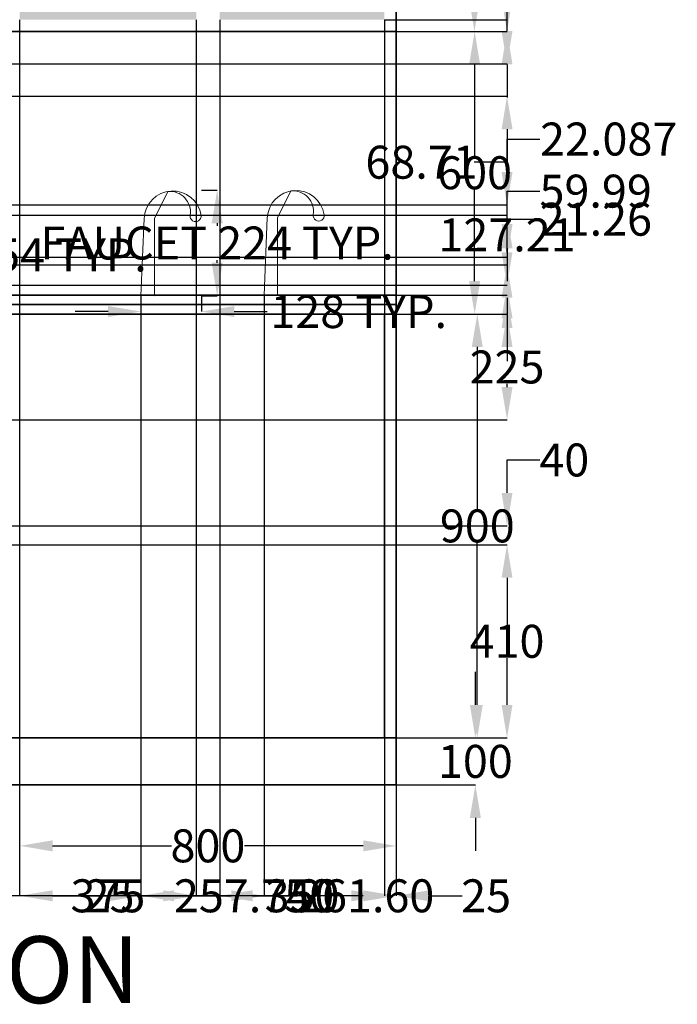
# Model space of a CAD drawing. Units: inches. Extents: x 600 to 5582, y -464 to 3142.
# Tile 8 of 9: x 4185 to 5582, y -464 to 1627. Entities that reach past the tile are written whole.
import ezdxf

# ---------------------------------------------------------------- set-up
doc = ezdxf.new("R2010")
doc.units = ezdxf.units.IN
doc.header["$MEASUREMENT"] = 0
for name, color, linetype, lineweight in [('A-ANNO-DIMS', 2, 'Continuous', 18), ('A-ANNO-TEXT', 7, 'Continuous', 25), ('A-ELEV', 7, 'Continuous', 35), ('A-ELEV-PATT', 252, 'Continuous', 13), ('A-FLOR-FIXT', 8, 'Continuous', 18)]:
    doc.layers.add(name, color=color, linetype=linetype, lineweight=lineweight)
doc.styles.get("Standard").update_dxf_attribs({"font": 'arial.ttf'})
doc.dimstyles.get("Standard").update_dxf_attribs({"dimtxt": 70, "dimasz": 70, "dimexe": 0.18, "dimexo": 0.0625, "dimgap": 0.09, "dimtad": 0, "dimtih": 1, "dimtoh": 1, "dimdec": 0, "dimzin": 0, "dimdsep": 46, "dimtxsty": 'Standard', "dimcen": 0.09, "dimadec": 0, "dimazin": 0, "dimtfac": 1, "dimtdec": 0, "dimtofl": 0, "dimtmove": 0, "dimatfit": 3, "dimfxl": 1, "dimtolj": 1, "dimtzin": 0, "dimarcsym": 0})

# ---------------------------------------------------------------- blocks, each defined once
blk = doc.blocks.new('*D2')
at = {"layer": 'A-ANNO-DIMS', "color": 0, "lineweight": -2, "transparency": 16777216}
for p, q in [((5152.9, 172.4), (5152.9, 242.4)), ((4984.8, 102.4), (5153.1, 102.4)), ((4984.8, 2.4), (5153.1, 2.4)), ((5152.9, -67.6), (5152.9, -137.6))]:
    blk.add_line(p, q, dxfattribs=at)
at = {"layer": 'A-ANNO-DIMS', "color": 0, "transparency": 16777216}
for points in [[(5141.2, 172.4), (5164.6, 172.4), (5152.9, 102.4)], [(5141.2, -67.6), (5164.6, -67.6), (5152.9, 2.4)]]:
    blk.add_solid(points, dxfattribs=at)
at = {"layer": 'Defpoints', "color": 0, "transparency": 16777216}
for p in [(4984.7, 102.4), (4984.7, 2.4), (5152.9, 2.4)]:
    blk.add_point(p, dxfattribs=at)
at = {"layer": 'A-ANNO-DIMS', "color": 0, "transparency": 16777216, "insert": (5152.9, 52.4), "char_height": 70, "attachment_point": 5}
blk.add_mtext('\\A1;100', dxfattribs=at)
blk = doc.blocks.new('*D3')
at = {"layer": 'A-ANNO-DIMS', "color": 0, "lineweight": -2, "transparency": 16777216}
for p, q in [((4984.8, 1002.4), (5157.2, 1002.4)), ((5157, 932.4), (5157, 588.3)), ((5157, 172.4), (5157, 516.6)), ((4984.8, 102.4), (5157.2, 102.4))]:
    blk.add_line(p, q, dxfattribs=at)
at = {"layer": 'A-ANNO-DIMS', "color": 0, "transparency": 16777216}
for points in [[(5145.3, 932.4), (5168.6, 932.4), (5157, 1002.4)], [(5145.3, 172.4), (5168.6, 172.4), (5157, 102.4)]]:
    blk.add_solid(points, dxfattribs=at)
at = {"layer": 'Defpoints', "color": 0, "transparency": 16777216}
for p in [(4984.7, 1002.4), (5157, 1002.4), (4984.7, 102.4)]:
    blk.add_point(p, dxfattribs=at)
at = {"layer": 'A-ANNO-DIMS', "color": 0, "transparency": 16777216, "insert": (5157, 552.4), "char_height": 70, "attachment_point": 5}
blk.add_mtext('\\A1;900', dxfattribs=at)
blk = doc.blocks.new('*D4')
at = {"layer": 'A-ANNO-DIMS', "color": 0, "lineweight": -2, "transparency": 16777216}
for p, q in [((4984.8, 1602.4), (5151.6, 1602.4)), ((5151.4, 1532.4), (5151.4, 1338.3)), ((5151.4, 1072.4), (5151.4, 1266.6)), ((4984.8, 1002.4), (5151.6, 1002.4))]:
    blk.add_line(p, q, dxfattribs=at)
at = {"layer": 'A-ANNO-DIMS', "color": 0, "transparency": 16777216}
for points in [[(5139.7, 1532.4), (5163.1, 1532.4), (5151.4, 1602.4)], [(5139.7, 1072.4), (5163.1, 1072.4), (5151.4, 1002.4)]]:
    blk.add_solid(points, dxfattribs=at)
at = {"layer": 'Defpoints', "color": 0, "transparency": 16777216}
for p in [(4984.7, 1602.4), (4984.7, 1002.4), (5151.4, 1002.4)]:
    blk.add_point(p, dxfattribs=at)
at = {"layer": 'A-ANNO-DIMS', "color": 0, "transparency": 16777216, "insert": (5151.4, 1302.4), "char_height": 70, "attachment_point": 5}
blk.add_mtext('\\A1;600', dxfattribs=at)
blk = doc.blocks.new('*D5')
at = {"layer": 'A-ANNO-DIMS', "color": 0, "lineweight": -2, "transparency": 16777216}
for p, q in [((4984.8, 2352.4), (5151.2, 2352.4)), ((5151, 2282.4), (5151, 2013.3)), ((5151, 1672.4), (5151, 1941.6)), ((4984.8, 1602.4), (5151.2, 1602.4))]:
    blk.add_line(p, q, dxfattribs=at)
at = {"layer": 'A-ANNO-DIMS', "color": 0, "transparency": 16777216}
for points in [[(5139.4, 2282.4), (5162.7, 2282.4), (5151, 2352.4)], [(5139.4, 1672.4), (5162.7, 1672.4), (5151, 1602.4)]]:
    blk.add_solid(points, dxfattribs=at)
at = {"layer": 'Defpoints', "color": 0, "transparency": 16777216}
for p in [(4984.7, 2352.4), (4984.7, 1602.4), (5151, 1602.4)]:
    blk.add_point(p, dxfattribs=at)
at = {"layer": 'A-ANNO-DIMS', "color": 0, "transparency": 16777216, "insert": (5151, 1977.4), "char_height": 70, "attachment_point": 5}
blk.add_mtext('\\A1;750', dxfattribs=at)
blk = doc.blocks.new('*D14')
at = {"layer": 'A-ANNO-DIMS', "color": 0, "lineweight": -2, "transparency": 16777216}
for p, q in [((4184.7, 2.4), (4184.7, -127.2)), ((4984.7, 2.4), (4984.7, -127.2)), ((4254.7, -127), (4507.4, -127)), ((4914.7, -127), (4662.1, -127))]:
    blk.add_line(p, q, dxfattribs=at)
at = {"layer": 'A-ANNO-DIMS', "color": 0, "transparency": 16777216}
for points in [[(4254.7, -115.3), (4254.7, -138.7), (4184.7, -127)], [(4914.7, -115.3), (4914.7, -138.7), (4984.7, -127)]]:
    blk.add_solid(points, dxfattribs=at)
at = {"layer": 'Defpoints', "color": 0, "transparency": 16777216}
for p in [(4184.7, 2.4), (4984.7, 2.4), (4984.7, -127)]:
    blk.add_point(p, dxfattribs=at)
at = {"layer": 'A-ANNO-DIMS', "color": 0, "transparency": 16777216, "insert": (4584.7, -127), "char_height": 70, "attachment_point": 5}
blk.add_mtext('\\A1;800', dxfattribs=at)
blk = doc.blocks.new('FAUCET')
blk.add_lwpolyline([(0.1, 0.4), (6.9, 164.5, -0.907043), (127.6, 171.3, -1.166611), (104.6, 171.3, 0.489908), (56.8, 221.8), (28.6, 164.5), (28.6, 0.4), (0.1, 1.6)], format="xyb")
blk = doc.blocks.new('*D17')
at = {"layer": 'A-ANNO-DIMS', "color": 0, "lineweight": -2, "transparency": 16777216}
for p, q in [((3196.2, 1104.9), (3196.2, 1128.1)), ((3266.2, 1127.9), (3279.8, 1127.9)), ((3349.8, 1104.9), (3349.8, 1128.1)), ((3349.8, 1127.9), (3419.8, 1127.9))]:
    blk.add_line(p, q, dxfattribs=at)
at = {"layer": 'A-ANNO-DIMS', "color": 0, "transparency": 16777216}
for points in [[(3266.2, 1139.5), (3266.2, 1116.2), (3196.2, 1127.9)], [(3279.8, 1139.5), (3279.8, 1116.2), (3349.8, 1127.9)]]:
    blk.add_solid(points, dxfattribs=at)
at = {"layer": 'Defpoints', "color": 0, "transparency": 16777216}
for p in [(3349.8, 1127.9), (3196.2, 1104.9), (3349.8, 1104.9)]:
    blk.add_point(p, dxfattribs=at)
at = {"layer": 'A-ANNO-DIMS', "color": 0, "transparency": 16777216, "insert": (3955.1, 1127.9), "char_height": 70, "attachment_point": 5}
blk.add_mtext('\\A1;HOB BURNER 154 TYP.', dxfattribs=at)
blk = doc.blocks.new('*D19')
at = {"layer": 'A-ANNO-DIMS', "color": 0, "lineweight": -2, "transparency": 16777216}
for p, q in [((4570.8, 1265.2), (4604.5, 1265.2)), ((4604.3, 1195.2), (4604.3, 1189.5)), ((4604.3, 1111.2), (4604.3, 1117)), ((4570.8, 1041.2), (4604.5, 1041.2))]:
    blk.add_line(p, q, dxfattribs=at)
at = {"layer": 'A-ANNO-DIMS', "color": 0, "transparency": 16777216}
for points in [[(4592.7, 1195.2), (4616, 1195.2), (4604.3, 1265.2)], [(4592.7, 1111.2), (4616, 1111.2), (4604.3, 1041.2)]]:
    blk.add_solid(points, dxfattribs=at)
at = {"layer": 'Defpoints', "color": 0, "transparency": 16777216}
for p in [(4570.7, 1265.2), (4604.3, 1265.2), (4570.7, 1041.2)]:
    blk.add_point(p, dxfattribs=at)
at = {"layer": 'A-ANNO-DIMS', "color": 0, "transparency": 16777216, "insert": (4604.3, 1153.2), "char_height": 70, "attachment_point": 5}
blk.add_mtext('\\A1;FAUCET 224 TYP.', dxfattribs=at)
blk = doc.blocks.new('*D20')
at = {"layer": 'A-ANNO-DIMS', "color": 0, "lineweight": -2, "transparency": 16777216}
for p, q in [((4442.5, 1041.2), (4442.5, 1007.5)), ((4570.7, 1041.2), (4570.7, 1007.5)), ((4372.5, 1007.6), (4302.5, 1007.6)), ((4640.7, 1007.6), (4710.7, 1007.6))]:
    blk.add_line(p, q, dxfattribs=at)
at = {"layer": 'A-ANNO-DIMS', "color": 0, "transparency": 16777216}
for points in [[(4372.5, 1019.3), (4372.5, 996), (4442.5, 1007.6)], [(4640.7, 1019.3), (4640.7, 996), (4570.7, 1007.6)]]:
    blk.add_solid(points, dxfattribs=at)
at = {"layer": 'Defpoints', "color": 0, "transparency": 16777216}
for p in [(4442.5, 1041.2), (4570.7, 1041.2), (4570.7, 1007.6)]:
    blk.add_point(p, dxfattribs=at)
at = {"layer": 'A-ANNO-DIMS', "color": 0, "transparency": 16777216, "insert": (4905.1, 1007.6), "char_height": 70, "attachment_point": 5}
blk.add_mtext('\\A1;128 TYP.', dxfattribs=at)
blk = doc.blocks.new('*D21')
at = {"layer": 'A-ANNO-DIMS', "color": 0, "lineweight": -2, "transparency": 16777216}
for p, q in [((1384.7, 2.4), (1384.7, -233.3)), ((4984.7, 2.4), (4984.7, -233.3)), ((1454.7, -233.1), (3080.3, -233.1)), ((4914.7, -233.1), (3289.2, -233.1))]:
    blk.add_line(p, q, dxfattribs=at)
at = {"layer": 'A-ANNO-DIMS', "color": 0, "transparency": 16777216}
for points in [[(1454.7, -221.4), (1454.7, -244.7), (1384.7, -233.1)], [(4914.7, -221.4), (4914.7, -244.7), (4984.7, -233.1)]]:
    blk.add_solid(points, dxfattribs=at)
at = {"layer": 'Defpoints', "color": 0, "transparency": 16777216}
for p in [(1384.7, 2.4), (4984.7, 2.4), (4984.7, -233.1)]:
    blk.add_point(p, dxfattribs=at)
at = {"layer": 'A-ANNO-DIMS', "color": 0, "transparency": 16777216, "insert": (3184.7, -233.1), "char_height": 70, "attachment_point": 5}
blk.add_mtext('\\A1;3600', dxfattribs=at)
blk = doc.blocks.new('*D30')
at = {"layer": 'A-ANNO-DIMS', "color": 0, "lineweight": -2, "transparency": 16777216}
for p, q in [((4159.7, 1627.4), (4159.7, -233.3)), ((4184.7, 1627.4), (4184.7, -233.3)), ((4089.7, -233.1), (4019.7, -233.1)), ((4254.7, -233.1), (4324.7, -233.1))]:
    blk.add_line(p, q, dxfattribs=at)
at = {"layer": 'A-ANNO-DIMS', "color": 0, "transparency": 16777216}
for points in [[(4089.7, -221.4), (4089.7, -244.7), (4159.7, -233.1)], [(4254.7, -221.4), (4254.7, -244.7), (4184.7, -233.1)]]:
    blk.add_solid(points, dxfattribs=at)
at = {"layer": 'Defpoints', "color": 0, "transparency": 16777216}
for p in [(4159.7, 1627.4), (4184.7, 1627.4), (4184.7, -233.1)]:
    blk.add_point(p, dxfattribs=at)
at = {"layer": 'A-ANNO-DIMS', "color": 0, "transparency": 16777216, "insert": (4375.8, -233.1), "char_height": 70, "attachment_point": 5}
blk.add_mtext('\\A1;25', dxfattribs=at)
blk = doc.blocks.new('*D31')
at = {"layer": 'A-ANNO-DIMS', "color": 0, "lineweight": -2, "transparency": 16777216}
for p, q in [((4184.7, 1627.4), (4184.7, -233.3)), ((4559.7, 1627.4), (4559.7, -233.3)), ((4254.7, -233.1), (4294.6, -233.1)), ((4489.7, -233.1), (4449.9, -233.1))]:
    blk.add_line(p, q, dxfattribs=at)
at = {"layer": 'A-ANNO-DIMS', "color": 0, "transparency": 16777216}
for points in [[(4254.7, -221.4), (4254.7, -244.7), (4184.7, -233.1)], [(4489.7, -221.4), (4489.7, -244.7), (4559.7, -233.1)]]:
    blk.add_solid(points, dxfattribs=at)
at = {"layer": 'Defpoints', "color": 0, "transparency": 16777216}
for p in [(4184.7, 1627.4), (4559.7, 1627.4), (4559.7, -233.1)]:
    blk.add_point(p, dxfattribs=at)
at = {"layer": 'A-ANNO-DIMS', "color": 0, "transparency": 16777216, "insert": (4372.2, -233.1), "char_height": 70, "attachment_point": 5}
blk.add_mtext('\\A1;375', dxfattribs=at)
blk = doc.blocks.new('*D32')
at = {"layer": 'A-ANNO-DIMS', "color": 0, "lineweight": -2, "transparency": 16777216}
for p, q in [((4559.7, 1627.4), (4559.7, -233.3)), ((4609.7, 1627.4), (4609.7, -233.3)), ((4489.7, -233.1), (4419.7, -233.1)), ((4679.7, -233.1), (4749.7, -233.1))]:
    blk.add_line(p, q, dxfattribs=at)
at = {"layer": 'A-ANNO-DIMS', "color": 0, "transparency": 16777216}
for points in [[(4489.7, -221.4), (4489.7, -244.7), (4559.7, -233.1)], [(4679.7, -221.4), (4679.7, -244.7), (4609.7, -233.1)]]:
    blk.add_solid(points, dxfattribs=at)
at = {"layer": 'Defpoints', "color": 0, "transparency": 16777216}
for p in [(4559.7, 1627.4), (4609.7, 1627.4), (4609.7, -233.1)]:
    blk.add_point(p, dxfattribs=at)
at = {"layer": 'A-ANNO-DIMS', "color": 0, "transparency": 16777216, "insert": (4799.9, -233.1), "char_height": 70, "attachment_point": 5}
blk.add_mtext('\\A1;50', dxfattribs=at)
blk = doc.blocks.new('*D33')
at = {"layer": 'A-ANNO-DIMS', "color": 0, "lineweight": -2, "transparency": 16777216}
for p, q in [((4609.7, 1627.4), (4609.7, -233.3)), ((4959.7, 1627.4), (4959.7, -233.3)), ((4679.7, -233.1), (4707.5, -233.1)), ((4889.7, -233.1), (4862, -233.1))]:
    blk.add_line(p, q, dxfattribs=at)
at = {"layer": 'A-ANNO-DIMS', "color": 0, "transparency": 16777216}
for points in [[(4679.7, -221.4), (4679.7, -244.7), (4609.7, -233.1)], [(4889.7, -221.4), (4889.7, -244.7), (4959.7, -233.1)]]:
    blk.add_solid(points, dxfattribs=at)
at = {"layer": 'Defpoints', "color": 0, "transparency": 16777216}
for p in [(4609.7, 1627.4), (4959.7, 1627.4), (4959.7, -233.1)]:
    blk.add_point(p, dxfattribs=at)
at = {"layer": 'A-ANNO-DIMS', "color": 0, "transparency": 16777216, "insert": (4784.7, -233.1), "char_height": 70, "attachment_point": 5}
blk.add_mtext('\\A1;350', dxfattribs=at)
blk = doc.blocks.new('*D34')
at = {"layer": 'A-ANNO-DIMS', "color": 0, "lineweight": -2, "transparency": 16777216}
for p, q in [((4959.7, 1627.4), (4959.7, -233.3)), ((4984.7, 1602.4), (4984.7, -233.3)), ((4889.7, -233.1), (4819.7, -233.1)), ((5054.7, -233.1), (5124.7, -233.1))]:
    blk.add_line(p, q, dxfattribs=at)
at = {"layer": 'A-ANNO-DIMS', "color": 0, "transparency": 16777216}
for points in [[(4889.7, -221.4), (4889.7, -244.7), (4959.7, -233.1)], [(5054.7, -221.4), (5054.7, -244.7), (4984.7, -233.1)]]:
    blk.add_solid(points, dxfattribs=at)
at = {"layer": 'Defpoints', "color": 0, "transparency": 16777216}
for p in [(4959.7, 1627.4), (4984.7, 1602.4), (4984.7, -233.1)]:
    blk.add_point(p, dxfattribs=at)
at = {"layer": 'A-ANNO-DIMS', "color": 0, "transparency": 16777216, "insert": (5175.8, -233.1), "char_height": 70, "attachment_point": 5}
blk.add_mtext('\\A1;25', dxfattribs=at)
blk = doc.blocks.new('*D35')
at = {"layer": 'A-ANNO-DIMS', "color": 0, "lineweight": -2, "transparency": 16777216}
for p, q in [((5220.2, 1697.4), (5220.2, 1767.4)), ((5220.2, 1767.4), (5290.2, 1767.4)), ((4959.8, 1627.4), (5220.4, 1627.4)), ((4984.8, 1602.4), (5220.4, 1602.4)), ((5220.2, 1532.4), (5220.2, 1462.4))]:
    blk.add_line(p, q, dxfattribs=at)
at = {"layer": 'A-ANNO-DIMS', "color": 0, "transparency": 16777216}
for points in [[(5208.6, 1697.4), (5231.9, 1697.4), (5220.2, 1627.4)], [(5208.6, 1532.4), (5231.9, 1532.4), (5220.2, 1602.4)]]:
    blk.add_solid(points, dxfattribs=at)
at = {"layer": 'Defpoints', "color": 0, "transparency": 16777216}
for p in [(4959.7, 1627.4), (5220.2, 1627.4), (4984.7, 1602.4)]:
    blk.add_point(p, dxfattribs=at)
at = {"layer": 'A-ANNO-DIMS', "color": 0, "transparency": 16777216, "insert": (5341.3, 1767.4), "char_height": 70, "attachment_point": 5}
blk.add_mtext('\\A1;25', dxfattribs=at)
blk = doc.blocks.new('*D36')
at = {"layer": 'A-ANNO-DIMS', "color": 0, "lineweight": -2, "transparency": 16777216}
for p, q in [((4959.8, 1977.4), (5220.4, 1977.4)), ((5220.2, 1907.4), (5220.2, 1838.3)), ((5220.2, 1697.4), (5220.2, 1766.6)), ((4959.8, 1627.4), (5220.4, 1627.4))]:
    blk.add_line(p, q, dxfattribs=at)
at = {"layer": 'A-ANNO-DIMS', "color": 0, "transparency": 16777216}
for points in [[(5208.6, 1907.4), (5231.9, 1907.4), (5220.2, 1977.4)], [(5208.6, 1697.4), (5231.9, 1697.4), (5220.2, 1627.4)]]:
    blk.add_solid(points, dxfattribs=at)
at = {"layer": 'Defpoints', "color": 0, "transparency": 16777216}
for p in [(4959.7, 1977.4), (5220.2, 1977.4), (4959.7, 1627.4)]:
    blk.add_point(p, dxfattribs=at)
at = {"layer": 'A-ANNO-DIMS', "color": 0, "transparency": 16777216, "insert": (5220.2, 1802.4), "char_height": 70, "attachment_point": 5}
blk.add_mtext('\\A1;350', dxfattribs=at)
blk = doc.blocks.new('*D47')
at = {"layer": 'A-ANNO-DIMS', "color": 0, "lineweight": -2, "transparency": 16777216}
for p, q in [((3384.8, 1002.4), (5220.4, 1002.4)), ((5220.2, 932.4), (5220.2, 925.8)), ((5220.2, 847.4), (5220.2, 854.1)), ((3384.8, 777.4), (5220.4, 777.4))]:
    blk.add_line(p, q, dxfattribs=at)
at = {"layer": 'A-ANNO-DIMS', "color": 0, "transparency": 16777216}
for points in [[(5208.6, 932.4), (5231.9, 932.4), (5220.2, 1002.4)], [(5208.6, 847.4), (5231.9, 847.4), (5220.2, 777.4)]]:
    blk.add_solid(points, dxfattribs=at)
at = {"layer": 'Defpoints', "color": 0, "transparency": 16777216}
for p in [(3384.7, 1002.4), (5220.2, 1002.4), (3384.7, 777.4)]:
    blk.add_point(p, dxfattribs=at)
at = {"layer": 'A-ANNO-DIMS', "color": 0, "transparency": 16777216, "insert": (5220.2, 889.9), "char_height": 70, "attachment_point": 5}
blk.add_mtext('\\A1;225', dxfattribs=at)
blk = doc.blocks.new('*D56')
at = {"layer": 'A-ANNO-DIMS', "color": 0, "lineweight": -2, "transparency": 16777216}
for p, q in [((1884.8, 512.4), (5220.4, 512.4)), ((5220.2, 442.4), (5220.2, 343.3)), ((5220.2, 172.4), (5220.2, 271.6)), ((1884.8, 102.4), (5220.4, 102.4))]:
    blk.add_line(p, q, dxfattribs=at)
at = {"layer": 'A-ANNO-DIMS', "color": 0, "transparency": 16777216}
for points in [[(5208.6, 442.4), (5231.9, 442.4), (5220.2, 512.4)], [(5208.6, 172.4), (5231.9, 172.4), (5220.2, 102.4)]]:
    blk.add_solid(points, dxfattribs=at)
at = {"layer": 'Defpoints', "color": 0, "transparency": 16777216}
for p in [(1884.7, 512.4), (5220.2, 512.4), (1884.7, 102.4)]:
    blk.add_point(p, dxfattribs=at)
at = {"layer": 'A-ANNO-DIMS', "color": 0, "transparency": 16777216, "insert": (5220.2, 307.4), "char_height": 70, "attachment_point": 5}
blk.add_mtext('\\A1;410', dxfattribs=at)
blk = doc.blocks.new('*D57')
at = {"layer": 'A-ANNO-DIMS', "color": 0, "lineweight": -2, "transparency": 16777216}
for p, q in [((5220.2, 622.4), (5220.2, 692.4)), ((5220.2, 692.4), (5290.2, 692.4)), ((1884.8, 552.4), (5220.4, 552.4)), ((1884.8, 512.4), (5220.4, 512.4)), ((5220.2, 442.4), (5220.2, 372.4))]:
    blk.add_line(p, q, dxfattribs=at)
at = {"layer": 'A-ANNO-DIMS', "color": 0, "transparency": 16777216}
for points in [[(5208.6, 622.4), (5231.9, 622.4), (5220.2, 552.4)], [(5208.6, 442.4), (5231.9, 442.4), (5220.2, 512.4)]]:
    blk.add_solid(points, dxfattribs=at)
at = {"layer": 'Defpoints', "color": 0, "transparency": 16777216}
for p in [(1884.7, 552.4), (5220.2, 552.4), (1884.7, 512.4)]:
    blk.add_point(p, dxfattribs=at)
at = {"layer": 'A-ANNO-DIMS', "color": 0, "transparency": 16777216, "insert": (5341.8, 692.4), "char_height": 70, "attachment_point": 5}
blk.add_mtext('\\A1;40', dxfattribs=at)
blk = doc.blocks.new('*D61')
at = {"layer": 'A-ANNO-DIMS', "color": 0, "lineweight": -2, "transparency": 16777216}
for p, q in [((4637.7, 1954.9), (5220.4, 1954.9)), ((5220.2, 1884.9), (5220.2, 1814.5)), ((5220.2, 1672.4), (5220.2, 1742.8)), ((4984.8, 1602.4), (5220.4, 1602.4))]:
    blk.add_line(p, q, dxfattribs=at)
at = {"layer": 'A-ANNO-DIMS', "color": 0, "transparency": 16777216}
for points in [[(5208.6, 1884.9), (5231.9, 1884.9), (5220.2, 1954.9)], [(5208.6, 1672.4), (5231.9, 1672.4), (5220.2, 1602.4)]]:
    blk.add_solid(points, dxfattribs=at)
at = {"layer": 'Defpoints', "color": 0, "transparency": 16777216}
for p in [(4637.6, 1954.9), (5220.2, 1954.9), (4984.7, 1602.4)]:
    blk.add_point(p, dxfattribs=at)
at = {"layer": 'A-ANNO-DIMS', "color": 0, "transparency": 16777216, "insert": (5220.2, 1778.6), "char_height": 70, "attachment_point": 5}
blk.add_mtext('\\A1;352.44', dxfattribs=at)
blk = doc.blocks.new('*D66')
at = {"layer": 'A-ANNO-DIMS', "color": 0, "lineweight": -2, "transparency": 16777216}
for p, q in [((4442.5, 1041.2), (4442.5, -233.3)), ((4184.7, 1002.4), (4184.7, -233.3)), ((4254.7, -233.1), (4372.5, -233.1)), ((4442.5, -233.1), (4512.5, -233.1))]:
    blk.add_line(p, q, dxfattribs=at)
at = {"layer": 'A-ANNO-DIMS', "color": 0, "transparency": 16777216}
for points in [[(4254.7, -221.4), (4254.7, -244.7), (4184.7, -233.1)], [(4372.5, -221.4), (4372.5, -244.7), (4442.5, -233.1)]]:
    blk.add_solid(points, dxfattribs=at)
at = {"layer": 'Defpoints', "color": 0, "transparency": 16777216}
for p in [(4442.5, 1041.2), (4184.7, 1002.4), (4442.5, -233.1)]:
    blk.add_point(p, dxfattribs=at)
at = {"layer": 'A-ANNO-DIMS', "color": 0, "transparency": 16777216, "insert": (4658.3, -233.1), "char_height": 70, "attachment_point": 5}
blk.add_mtext('\\A1;257.74', dxfattribs=at)
blk = doc.blocks.new('*D67')
at = {"layer": 'A-ANNO-DIMS', "color": 0, "lineweight": -2, "transparency": 16777216}
for p, q in [((4442.5, 1041.2), (4442.5, -233.3)), ((4704.1, 1042.4), (4704.1, -233.3)), ((4512.5, -233.1), (4634.1, -233.1)), ((4704.1, -233.1), (4774.1, -233.1))]:
    blk.add_line(p, q, dxfattribs=at)
at = {"layer": 'A-ANNO-DIMS', "color": 0, "transparency": 16777216}
for points in [[(4512.5, -221.4), (4512.5, -244.7), (4442.5, -233.1)], [(4634.1, -221.4), (4634.1, -244.7), (4704.1, -233.1)]]:
    blk.add_solid(points, dxfattribs=at)
at = {"layer": 'Defpoints', "color": 0, "transparency": 16777216}
for p in [(4442.5, 1041.2), (4704.1, 1042.4), (4704.1, -233.1)]:
    blk.add_point(p, dxfattribs=at)
at = {"layer": 'A-ANNO-DIMS', "color": 0, "transparency": 16777216, "insert": (4920, -233.1), "char_height": 70, "attachment_point": 5}
blk.add_mtext('\\A1;261.60', dxfattribs=at)
blk = doc.blocks.new('*D69')
at = {"layer": 'A-ANNO-DIMS', "color": 0, "lineweight": -2, "transparency": 16777216}
for p, q in [((5220.2, 1304), (5220.2, 1374)), ((2777.3, 1234), (5220.4, 1234)), ((2777.3, 1106.8), (5220.4, 1106.8)), ((5220.2, 1036.8), (5220.2, 966.8))]:
    blk.add_line(p, q, dxfattribs=at)
at = {"layer": 'A-ANNO-DIMS', "color": 0, "transparency": 16777216}
for points in [[(5208.6, 1304), (5231.9, 1304), (5220.2, 1234)], [(5208.6, 1036.8), (5231.9, 1036.8), (5220.2, 1106.8)]]:
    blk.add_solid(points, dxfattribs=at)
at = {"layer": 'Defpoints', "color": 0, "transparency": 16777216}
for p in [(2777.3, 1234), (5220.2, 1234), (2777.3, 1106.8)]:
    blk.add_point(p, dxfattribs=at)
at = {"layer": 'A-ANNO-DIMS', "color": 0, "transparency": 16777216, "insert": (5220.2, 1170.4), "char_height": 70, "attachment_point": 5}
blk.add_mtext('\\A1;127.21', dxfattribs=at)
blk = doc.blocks.new('*D72')
at = {"layer": 'A-ANNO-DIMS', "color": 0, "lineweight": -2, "transparency": 16777216}
for p, q in [((5220.2, 1304), (5220.2, 1374)), ((5220.2, 1374), (5290.2, 1374)), ((2947.9, 1234), (5220.4, 1234)), ((2947.9, 1212), (5220.4, 1212)), ((5220.2, 1142), (5220.2, 1072))]:
    blk.add_line(p, q, dxfattribs=at)
at = {"layer": 'A-ANNO-DIMS', "color": 0, "transparency": 16777216}
for points in [[(5208.6, 1304), (5231.9, 1304), (5220.2, 1234)], [(5208.6, 1142), (5231.9, 1142), (5220.2, 1212)]]:
    blk.add_solid(points, dxfattribs=at)
at = {"layer": 'Defpoints', "color": 0, "transparency": 16777216}
for p in [(2947.8, 1234), (5220.2, 1234), (2947.8, 1212)]:
    blk.add_point(p, dxfattribs=at)
at = {"layer": 'A-ANNO-DIMS', "color": 0, "transparency": 16777216, "insert": (5436.2, 1374), "char_height": 70, "attachment_point": 5}
blk.add_mtext('\\A1;22.087', dxfattribs=at)
blk = doc.blocks.new('*D81')
at = {"layer": 'A-ANNO-DIMS', "color": 0, "lineweight": -2, "transparency": 16777216}
for p, q in [((5220.2, 1133.7), (5220.2, 1203.7)), ((5220.2, 1203.7), (5290.2, 1203.7)), ((2292.1, 1063.7), (5220.4, 1063.7)), ((2310.1, 1042.4), (5220.4, 1042.4)), ((5220.2, 972.4), (5220.2, 902.4))]:
    blk.add_line(p, q, dxfattribs=at)
at = {"layer": 'A-ANNO-DIMS', "color": 0, "transparency": 16777216}
for points in [[(5208.6, 1133.7), (5231.9, 1133.7), (5220.2, 1063.7)], [(5208.6, 972.4), (5231.9, 972.4), (5220.2, 1042.4)]]:
    blk.add_solid(points, dxfattribs=at)
at = {"layer": 'Defpoints', "color": 0, "transparency": 16777216}
for p in [(2292, 1063.7), (5220.2, 1063.7), (2310, 1042.4)]:
    blk.add_point(p, dxfattribs=at)
at = {"layer": 'A-ANNO-DIMS', "color": 0, "transparency": 16777216, "insert": (5409, 1203.7), "char_height": 70, "attachment_point": 5}
blk.add_mtext('\\A1;21.26', dxfattribs=at)
blk = doc.blocks.new('*D85')
at = {"layer": 'A-ANNO-DIMS', "color": 0, "lineweight": -2, "transparency": 16777216}
for p, q in [((5220.2, 1193.3), (5220.2, 1263.3)), ((5220.2, 1263.3), (5290.2, 1263.3)), ((2231.9, 1123.3), (5220.4, 1123.3)), ((2232.3, 1063.4), (5220.4, 1063.4)), ((5220.2, 993.4), (5220.2, 923.4))]:
    blk.add_line(p, q, dxfattribs=at)
at = {"layer": 'A-ANNO-DIMS', "color": 0, "transparency": 16777216}
for points in [[(5208.6, 1193.3), (5231.9, 1193.3), (5220.2, 1123.3)], [(5208.6, 993.4), (5231.9, 993.4), (5220.2, 1063.4)]]:
    blk.add_solid(points, dxfattribs=at)
at = {"layer": 'Defpoints', "color": 0, "transparency": 16777216}
for p in [(2231.8, 1123.3), (5220.2, 1123.3), (2232.2, 1063.4)]:
    blk.add_point(p, dxfattribs=at)
at = {"layer": 'A-ANNO-DIMS', "color": 0, "transparency": 16777216, "insert": (5408.5, 1263.3), "char_height": 70, "attachment_point": 5}
blk.add_mtext('\\A1;59.99', dxfattribs=at)
blk = doc.blocks.new('*D99')
at = {"layer": 'A-ANNO-DIMS', "color": 0, "lineweight": -2, "transparency": 16777216}
for p, q in [((5220.2, 1603.5), (5220.2, 1673.5)), ((2271, 1533.5), (5220.4, 1533.5)), ((2273, 1464.8), (5220.4, 1464.8)), ((5220.2, 1394.8), (5220.2, 1324.8)), ((5220.2, 1324.8), (5150.2, 1324.8))]:
    blk.add_line(p, q, dxfattribs=at)
at = {"layer": 'A-ANNO-DIMS', "color": 0, "transparency": 16777216}
for points in [[(5208.6, 1603.5), (5231.9, 1603.5), (5220.2, 1533.5)], [(5208.6, 1394.8), (5231.9, 1394.8), (5220.2, 1464.8)]]:
    blk.add_solid(points, dxfattribs=at)
at = {"layer": 'Defpoints', "color": 0, "transparency": 16777216}
for p in [(2271, 1533.5), (2272.9, 1464.8), (5220.2, 1464.8)]:
    blk.add_point(p, dxfattribs=at)
at = {"layer": 'A-ANNO-DIMS', "color": 0, "transparency": 16777216, "insert": (5038.6, 1324.8), "char_height": 70, "attachment_point": 5}
blk.add_mtext('\\A1;68.71', dxfattribs=at)

msp = doc.modelspace()

# ---------------------------------------------------------------- hatches: boundary and pattern name
at = {"layer": 'A-ELEV-PATT'}
h = msp.add_hatch(dxfattribs=at)
h.set_pattern_fill('CROSS', color=256, scale=100)
h.paths.add_polyline_path([(1759.7485, 2327.4212), (1409.7485, 2327.4212), (1409.7485, 1967.4212), (1759.7485, 1967.4212)])
h.paths.add_polyline_path([(1759.7485, 1952.4212), (1409.7485, 1952.4212), (1409.7485, 1567.4212), (1759.7485, 1567.4212)])
h.paths.add_polyline_path([(1759.7485, 1552.4212), (1409.7485, 1552.4212), (1409.7485, 1167.4212), (1759.7485, 1167.4212)])
h.paths.add_polyline_path([(1759.7485, 1152.4212), (1409.7485, 1152.4212), (1409.7485, 767.4212), (1759.7485, 767.4212)])
h.paths.add_polyline_path([(1759.7485, 752.4212), (1409.7485, 752.4212), (1409.7485, 367.4212), (1759.7485, 367.4212)])
h.paths.add_polyline_path([(1759.7485, 352.4212), (1409.7485, 352.4212), (1409.7485, 142.4212), (1759.7485, 142.4212)])
h.paths.add_polyline_path([(3759.7485, 1977.4212), (3409.7485, 1977.4212), (3409.7485, 1627.4212), (3759.7485, 1627.4212)])
h.paths.add_polyline_path([(3714.7508, 1954.858, -1), (3750.8891, 1954.858, -1)], flags=16)
h.paths.add_polyline_path([(3759.7485, 2327.4212), (3409.7485, 2327.4212), (3409.7485, 2002.4212), (3759.7485, 2002.4212)])
h.paths.add_polyline_path([(4159.7485, 2327.4212), (3809.7485, 2327.4212), (3809.7485, 2002.4212), (4159.7485, 2002.4212)])
h.paths.add_polyline_path([(4159.7485, 1977.4212), (3809.7485, 1977.4212), (3813.5467, 1954.858, -1), (3849.685, 1954.858, -1), (3813.5467, 1954.858), (3809.7485, 1627.4212), (4159.7485, 1627.4212)])
h.paths.add_polyline_path([(4559.7485, 2327.4212), (4184.7485, 2327.4212), (4184.7485, 2002.4212), (4559.7485, 2002.4212)])
h.paths.add_polyline_path([(4559.7485, 1977.4212), (4184.7485, 1977.4212), (4184.7485, 1627.4212), (4559.7485, 1627.4212)])
h.paths.add_polyline_path([(4517.0704, 1954.858, -1), (4553.2087, 1954.858, -1)], flags=16)
h.paths.add_polyline_path([(4959.7485, 2327.4212), (4609.7485, 2327.4212), (4609.7485, 2002.4212), (4959.7485, 2002.4212)])
h.paths.add_polyline_path([(4959.7485, 1977.4212), (4609.7485, 1977.4212), (4609.7485, 1627.4212), (4959.7485, 1627.4212)])
h.paths.add_polyline_path([(4619.5464, 1954.858, -1), (4655.6847, 1954.858, -1)], flags=16)

# ---------------------------------------------------------------- linework, layer by layer
at = {"layer": 'A-ELEV'}
for p, q in [((4984.7485, 1042.4212), (1784.7485, 1042.4212)), ((4984.7485, 1022.4212), (1784.7485, 1022.4212)), ((4984.7485, 1002.4212), (1784.7485, 1002.4212)), ((4959.7485, 102.4212), (4959.7485, 1002.4212)), ((4984.7485, 102.4212), (1384.7485, 102.4212))]:
    msp.add_line(p, q, dxfattribs=at)
msp.add_lwpolyline([(4984.7485, 2.4212), (4984.7485, 2752.4212), (1384.7485, 2752.4212), (1384.7485, 2.4212)], close=True, dxfattribs=at)
msp.add_lwpolyline([(4984.7485, 1602.4212), (3384.7485, 1602.4212), (3384.7485, 2352.4212), (3784.7485, 2352.4212)], dxfattribs=at)

# ---------------------------------------------------------------- block references
at = {"layer": 'A-FLOR-FIXT'}
for p in [(4442.398, 1040.8238), (4704, 1042)]:
    msp.add_blockref('FAUCET', p, dxfattribs=at)

# ---------------------------------------------------------------- texts
at = {"layer": 'A-ANNO-TEXT'}
msp.add_text('MODULAR KITCHEN ELEVATION', height=141.903549, dxfattribs=at).set_placement((1598.0156, -460.987))

# ---------------------------------------------------------------- dimensions: what is measured, and where the dimension line sits
at = {"layer": 'A-ANNO-DIMS'}
for base, p1, p2, override, picture, middle in [((5151.032, 1602.4212), (4984.7485, 2352.4212), (4984.7485, 1602.4212), {"dimclrd": 0, "dimclre": 0, "dimclrt": 0}, '*D5', (5151.032, 1977.4212)), ((5220.2485, 1977.4212), (4959.7485, 1627.4212), (4959.7485, 1977.4212), {"dimdec": 0, "dimlfac": 1, "dimrnd": 0, "dimzin": 0, "dimdsep": 46, "dimlunit": 2}, '*D36', (5220.2485, 1802.4212)), ((5220.2485, 1954.858), (4984.7485, 1602.4212), (4637.6155, 1954.858), {"dimdec": 2, "dimlfac": 1, "dimrnd": 0, "dimzin": 0, "dimdsep": 46, "dimlunit": 2}, '*D61', (5220.2485, 1778.6396)), ((5220.2485, 1627.4212), (4984.7485, 1602.4212), (4959.7485, 1627.4212), {"dimdec": 0, "dimlfac": 1, "dimrnd": 0, "dimzin": 0, "dimdsep": 46, "dimlunit": 2}, '*D35', (5341.3344, 1767.4212)), ((5220.2485, 1464.7817), (2270.9593, 1533.4874), (2272.9025, 1464.7817), {"dimdec": 2, "dimlfac": 1, "dimrnd": 0, "dimzin": 0, "dimdsep": 46, "dimlunit": 2}, '*D99', (5038.6169, 1324.7817)), ((5151.412, 1002.4212), (4984.7485, 1602.4212), (4984.7485, 1002.4212), {"dimclrd": 0, "dimclre": 0, "dimclrt": 0}, '*D4', (5151.412, 1302.4212)), ((5220.2485, 1234.0488), (2947.8448, 1211.9616), (2947.8448, 1234.0488), {"dimdec": 3, "dimlfac": 1, "dimrnd": 0, "dimzin": 0, "dimdsep": 46, "dimlunit": 2}, '*D72', (5436.2355, 1374.0488)), ((5220.2485, 1234.0488), (2777.2556, 1106.8415), (2777.2556, 1234.0488), {"dimdec": 2, "dimlfac": 1, "dimrnd": 0, "dimzin": 0, "dimdsep": 46, "dimlunit": 2}, '*D69', (5220.2485, 1170.4451)), ((5220.2485, 1123.3472), (2232.228, 1063.362), (2231.8275, 1123.3472), {"dimdec": 2, "dimlfac": 1, "dimrnd": 0, "dimzin": 0, "dimdsep": 46, "dimlunit": 2}, '*D85', (5408.5172, 1263.3472)), ((5220.2485, 1063.682), (2310.0444, 1042.4212), (2292.0448, 1063.682), {"dimdec": 2, "dimlfac": 1, "dimrnd": 0, "dimzin": 0, "dimdsep": 46, "dimlunit": 2}, '*D81', (5409.0186, 1203.682)), ((5220.2485, 1002.4212), (3384.7485, 777.4212), (3384.7485, 1002.4212), {"dimdec": 0, "dimlfac": 1, "dimrnd": 0, "dimzin": 0, "dimdsep": 46, "dimlunit": 2}, '*D47', (5220.2485, 889.9212)), ((5156.983, 1002.4212), (4984.7485, 102.4212), (4984.7485, 1002.4212), {"dimclrd": 0, "dimclre": 0, "dimclrt": 0}, '*D3', (5156.983, 552.4212)), ((5220.2485, 552.4212), (1884.7485, 512.4212), (1884.7485, 552.4212), {"dimdec": 0, "dimlfac": 1, "dimrnd": 0, "dimzin": 0, "dimdsep": 46, "dimlunit": 2}, '*D57', (5341.7641, 692.4212)), ((5220.2485, 512.4212), (1884.7485, 102.4212), (1884.7485, 512.4212), {"dimdec": 0, "dimlfac": 1, "dimrnd": 0, "dimzin": 0, "dimdsep": 46, "dimlunit": 2}, '*D56', (5220.2485, 307.4212)), ((5152.9126, 2.4212), (4984.7485, 102.4212), (4984.7485, 2.4212), {"dimclrd": 0, "dimclre": 0, "dimclrt": 0}, '*D2', (5152.9126, 52.4212))]:
    dim = msp.add_linear_dim(base=base, p1=p1, p2=p2, angle=90, dimstyle='Standard', override=override, dxfattribs=at)
    dim.commit()
    dim.dimension.update_dxf_attribs({"geometry": picture, "text_midpoint": middle})
for base, p1, p2, override, picture, middle in [((4184.7485, -233.0788), (4159.7485, 1627.4212), (4184.7485, 1627.4212), {"dimdec": 0, "dimlfac": 1, "dimrnd": 0, "dimzin": 0, "dimdsep": 46, "dimlunit": 2}, '*D30', (4375.8344, -233.0788)), ((4559.7485, -233.0788), (4184.7485, 1627.4212), (4559.7485, 1627.4212), {"dimdec": 0, "dimlfac": 1, "dimrnd": 0, "dimzin": 0, "dimdsep": 46, "dimlunit": 2}, '*D31', (4372.2485, -233.0788)), ((4609.7485, -233.0788), (4559.7485, 1627.4212), (4609.7485, 1627.4212), {"dimdec": 0, "dimlfac": 1, "dimrnd": 0, "dimzin": 0, "dimdsep": 46, "dimlunit": 2}, '*D32', (4799.8555, -233.0788)), ((4959.7485, -233.0788), (4609.7485, 1627.4212), (4959.7485, 1627.4212), {"dimdec": 0, "dimlfac": 1, "dimrnd": 0, "dimzin": 0, "dimdsep": 46, "dimlunit": 2}, '*D33', (4784.7485, -233.0788)), ((4984.7485, -233.0788), (4959.7485, 1627.4212), (4984.7485, 1602.4212), {"dimdec": 0, "dimlfac": 1, "dimrnd": 0, "dimzin": 0, "dimdsep": 46, "dimlunit": 2}, '*D34', (5175.8344, -233.0788)), ((4442.4879, -233.0788), (4184.7485, 1002.4212), (4442.4879, 1041.2449), {"dimdec": 2, "dimlfac": 1, "dimrnd": 0, "dimzin": 0, "dimdsep": 46, "dimlunit": 2}, '*D66', (4658.3316, -233.0788)), ((4704.0898, -233.0788), (4442.4879, 1041.2449), (4704.0898, 1042.4212), {"dimdec": 2, "dimlfac": 1, "dimrnd": 0, "dimzin": 0, "dimdsep": 46, "dimlunit": 2}, '*D67', (4919.9575, -233.0788)), ((4984.7485, -233.0788), (1384.7485, 2.4212), (4984.7485, 2.4212), {"dimdec": 0, "dimlfac": 1, "dimrnd": 0, "dimzin": 0, "dimdsep": 46, "dimlunit": 2}, '*D21', (3184.7485, -233.0788)), ((4984.7485, -126.996), (4184.7485, 2.4212), (4984.7485, 2.4212), {"dimclrd": 0, "dimclre": 0, "dimclrt": 0}, '*D14', (4584.7485, -126.996))]:
    dim = msp.add_linear_dim(base=base, p1=p1, p2=p2, dimstyle='Standard', override=override, dxfattribs=at)
    dim.commit()
    dim.dimension.update_dxf_attribs({"geometry": picture, "text_midpoint": middle})
for base, p1, p2, text, picture, middle in [((3349.7642, 1127.8808), (3196.2381, 1104.8519), (3349.7642, 1104.8519), 'HOB BURNER <> TYP.', '*D17', (3955.1203, 1127.8808)), ((4570.7426, 1007.6448), (4442.4879, 1041.2449), (4570.7426, 1041.2449), '<> TYP.', '*D20', (4905.0993, 1007.6448))]:
    dim = msp.add_linear_dim(base=base, p1=p1, p2=p2, text=text, dimstyle='Standard', override={"dimdec": 0, "dimrnd": 0, "dimzin": 0, "dimlunit": 2}, dxfattribs=at)
    dim.commit()
    dim.dimension.update_dxf_attribs({"geometry": picture, "text_midpoint": middle})
dim = msp.add_linear_dim(base=(4604.3428, 1265.246), p1=(4570.7426, 1041.2449), p2=(4570.7426, 1265.246), angle=90, text='FAUCET <> TYP.', dimstyle='Standard', override={"dimdec": 0, "dimrnd": 0, "dimzin": 0, "dimlunit": 2}, dxfattribs=at)
dim.commit()
dim.dimension.update_dxf_attribs({"geometry": '*D19', "text_midpoint": (4604.3428, 1153.2455)})

doc.saveas('drawing.dxf')
